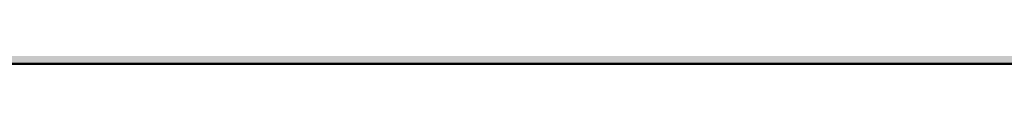
# Model space of a CAD drawing. Units: millimetres. Extents: x 0 to 2267, y 0 to 1823.
# Tile 235 of 256: x 1842.748 to 1843.095, y 1127.4171 to 1127.4171. Entities that reach past the tile are written whole.
import ezdxf

# ---------------------------------------------------------------- set-up
doc = ezdxf.new("R2010")
doc.units = ezdxf.units.MM
doc.header["$MEASUREMENT"] = 0
for name, color, linetype, lineweight in [('M-DIMS', 2, 'Continuous', 25), ('M-HATC', 252, 'Continuous', 18), ('M-OUTL', 7, 'Continuous', 50)]:
    doc.layers.add(name, color=color, linetype=linetype, lineweight=lineweight)
doc.styles.get("Standard").update_dxf_attribs({"font": 'arial.ttf'})
doc.dimstyles.get("Standard").update_dxf_attribs({"dimtxt": 7, "dimasz": 4, "dimexe": 0.18, "dimexo": 0.0625, "dimgap": 0.09, "dimtad": 0, "dimdec": 0, "dimzin": 0, "dimdsep": 46, "dimtxsty": 'Standard', "dimcen": 0.09, "dimadec": 0, "dimazin": 0, "dimtfac": 1, "dimtdec": 0, "dimtofl": 0, "dimtmove": 0, "dimatfit": 3, "dimfxl": 1, "dimtolj": 1, "dimtzin": 0, "dimarcsym": 0})

# ---------------------------------------------------------------- blocks, each defined once
blk = doc.blocks.new('*D1')
at = {"layer": 'Defpoints', "color": 0, "transparency": 16777216}
for p in [(1593.42891, 1127.41706), (1843.42891, 1127.41706), (1843.42891, 955.62775)]:
    blk.add_point(p, dxfattribs=at)
at = {"layer": 'M-DIMS', "color": 0, "lineweight": -2, "transparency": 16777216}
for p, q in [((1593.42891, 1127.35456), (1593.42891, 955.44775)), ((1843.42891, 1127.35456), (1843.42891, 955.44775)), ((1597.42891, 955.62775), (1710.55821, 955.62775)), ((1839.42891, 955.62775), (1726.2996, 955.62775))]:
    blk.add_line(p, q, dxfattribs=at)
at = {"layer": 'M-DIMS', "color": 0, "transparency": 16777216}
for points in [[(1597.42891, 956.29442), (1597.42891, 954.96109), (1593.42891, 955.62775)], [(1839.42891, 956.29442), (1839.42891, 954.96109), (1843.42891, 955.62775)]]:
    blk.add_solid(points, dxfattribs=at)
at = {"layer": 'M-DIMS', "color": 0, "transparency": 16777216, "insert": (1718.42891, 955.62775), "char_height": 7, "attachment_point": 5}
blk.add_mtext('\\A1;250', dxfattribs=at)

msp = doc.modelspace()

# ---------------------------------------------------------------- hatches: boundary and pattern name
at = {"layer": 'M-HATC'}
h = msp.add_hatch(color=256, dxfattribs=at)
h.dxf.hatch_style = 1
h.paths.add_polyline_path([(2042.88863, 1580.17963), (2055.77105, 1593.06204), (1381.08677, 1593.06204), (1393.96918, 1580.17963), (1374.08597, 1560.29642), (2062.77184, 1560.29642)])
h.paths.add_polyline_path([(1843.42891, 1201.32971), (1843.42891, 1227.24746), (1593.42891, 1227.24746), (1593.42891, 1201.32971, -0.228274), (1574.59893, 1162.23457), (1530.92891, 1127.41706), (1905.92891, 1127.41706), (1862.25888, 1162.23457, -0.228274)])

# ---------------------------------------------------------------- linework, layer by layer
at = {"layer": 'M-OUTL'}
msp.add_line((1530.92891, 1127.41706), (1905.92891, 1127.41706), dxfattribs=at)

# ---------------------------------------------------------------- dimensions: what is measured, and where the dimension line sits
at = {"layer": 'M-DIMS'}
dim = msp.add_linear_dim(base=(1843.42891, 955.62775), p1=(1593.42891, 1127.41706), p2=(1843.42891, 1127.41706), dimstyle='Standard', override={"dimclrd": 0, "dimclre": 0, "dimclrt": 0}, dxfattribs=at)
dim.commit()
dim.dimension.update_dxf_attribs({"geometry": '*D1', "text_midpoint": (1718.42891, 955.62775)})

doc.saveas('drawing.dxf')
